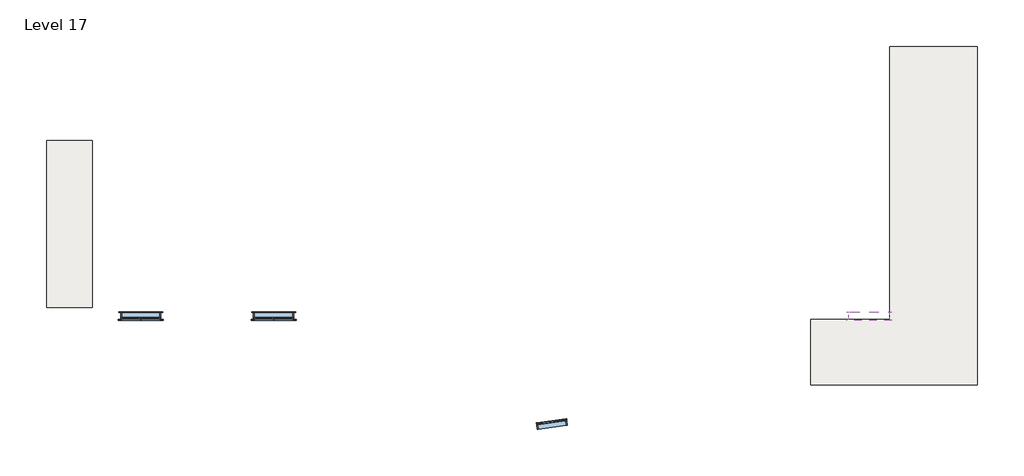
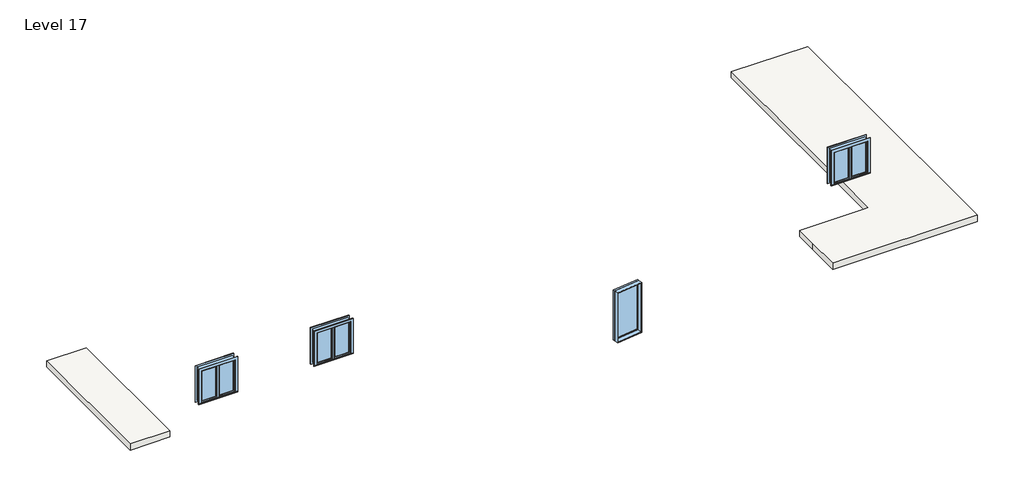
# One storey: 4 windows, 2 slabs.
"""IFC4 building model written with IfcOpenShell, lengths in millimetres."""

from ifc_helpers import new_model, si_unit, frame, origin, place, context, project, spatial, polyline, outline, extrude, transform, mapped, element, save
from components import window_0862ab64, window_9a779fa2

model = new_model("IFC4")

# Units and contexts
model_context = context("Model", 3, world=origin())
ifc_project = project(units=[si_unit("LENGTHUNIT", "METRE", prefix="MILLI")], contexts=[model_context])

# Site, building, storey
site = spatial("IfcSite", under=ifc_project)
building = spatial("IfcBuilding", under=site)
storey = spatial("IfcBuildingStorey", under=building, Name="Level 17", Elevation=26212.8)

# Slabs
placement = place(None, origin())
element("IfcSlab", 1, ObjectType="9\"", at=placement, inside=storey, context=model_context, shape_type="SweptSolid", body=[
    extrude(outline(polyline([(-17972.8272291, -8690.0239591), (-16601.2272291, -8690.0239591), (-16601.2272291, -13719.2239591), (-17972.8272291, -13719.2239591), (-17972.8272291, -8690.0239591)])), frame((0.0, 0.0, 25984.2), z_axis=(0.0, 0.0, 1.0), x_axis=(1.0, 0.0, 0.0)), (0.0, 0.0, 1.0), 228.6),
])
element("IfcSlab", 2, ObjectType="9\"", at=placement, inside=storey, context=model_context, shape_type="SweptSolid", body=[
    extrude(outline(polyline([(5046.5618272, -14840.0808221), (5046.5618272, -14078.0808221), (7230.9618272, -14078.0808221), (7434.1618272, -14078.0808221), (7434.1618272, -5848.4808221), (10075.7618272, -5848.4808221), (10075.7618272, -14840.0808221), (10075.7618272, -16059.2808221), (5046.5618272, -16059.2808221), (5046.5618272, -14840.0808221)])), frame((0.0, 0.0, 25984.2), z_axis=(0.0, 0.0, 1.0), x_axis=(1.0, 0.0, 0.0)), (0.0, 0.0, 1.0), 228.6),
])

# Windows
window_shape = window_0862ab64(model_context)
element("IfcWindow", 3, ObjectType="Casement Dbl with Trim : 48\" x 48\"", at=placement, inside=storey, context=model_context, shape_type="MappedRepresentation", body=[
    mapped(window_shape, transform((-15134.7505427, -13957.4308221, 26212.8), x_axis=(-1.0, 0.0, 0.0), y_axis=(0.0, -1.0, 0.0), z_axis=(0.0, 0.0, 1.0))),
])
element("IfcWindow", 4, ObjectType="Casement Dbl with Trim : 48\" x 48\"", at=placement, inside=storey, context=model_context, shape_type="MappedRepresentation", body=[
    mapped(window_shape, transform((-11129.6382271, -13957.4308221, 26212.8), x_axis=(-1.0, 0.0, 0.0), y_axis=(0.0, -1.0, 0.0), z_axis=(0.0, 0.0, 1.0))),
])
element("IfcWindow", 5, ObjectType="Casement Dbl with Trim : 48\" x 48\"", at=placement, inside=storey, context=model_context, shape_type="MappedRepresentation", body=[
    mapped(window_shape, transform((6810.8494573, -13957.4308221, 26558.0136494), x_axis=(-1.0, 0.0, 0.0), y_axis=(0.0, -1.0, 0.0), z_axis=(0.0, 0.0, 1.0))),
])
window_2_shape = window_9a779fa2(model_context)
element("IfcWindow", 6, ObjectType="Fixed : 36\" x 72\"", at=placement, inside=storey, context=model_context, shape_type="MappedRepresentation", body=[
    mapped(window_2_shape, transform((-2706.5288562, -17230.3159241, 26668.6120119), x_axis=(0.9910941253485877, 0.133163188229773, 0.0), y_axis=(-0.133163188229773, 0.9910941253485877, 0.0), z_axis=(0.0, 0.0, 1.0))),
])

save(model, "model.ifc")

# Revit data of these elements
# Type "9\""
#   Assembly Code = "B1010"
#   Function = 0
#   Layers, outside or top first: 0' - 9" no material (function 1)
# Type "Casement Dbl with Trim : 48\" x 48\""
#   Type Mark = "10"
#   Construction Type Id = "GSP4R"
#   Assembly Code = "B2020100"
#   Analytic Construction = "1/8 in Pilkington single glazing"
#   Visual Light Transmittance = 0.9
#   Solar Heat Gain Coefficient = 0.78
#   Heat Transfer Coefficient (U) = 0.6496 BTU/(h·ft²·°F)
#   Height = 4' - 0"
#   Default Sill Height = 3' - 0"
#   Trim Projection - Ext. = 0' - 0 1/2"
#   Trim Projection - Int. = 0' - 0 3/4"
#   Trim Width - Exterior = 0' - 3 1/2"
#   Trim Width - Interior = 0' - 3 1/2"
#   Width = 4' - 0"
#   Window Inset = 0' - 0 3/4"
#   Define Thermal Properties by = 1
#   Glass Pane Material = Glass
#   Sash Material = Sash
#   Trim Exterior Material = Trim
#   Trim Interior Material = Trim
#   Wall Closure = (empty or 0)
# Type "Fixed : 36\" x 72\""
#   Type Mark = "9"
#   Construction Type Id = "GSP4R"
#   Assembly Code = "B2020100"
#   Analytic Construction = "1/8 in Pilkington single glazing"
#   Visual Light Transmittance = 0.9
#   Solar Heat Gain Coefficient = 0.78
#   Heat Transfer Coefficient (U) = 0.6496 BTU/(h·ft²·°F)
#   Height = 6' - 0"
#   Default Sill Height = 1' - 0"
#   Width = 3' - 0"
#   Window Inset = 0' - 0 3/4"
#   Define Thermal Properties by = 1
#   Glass Pane Material = Glass
#   Sash Material = Sash
#   Wall Closure = (empty or 0)
# Element 1 (IfcSlab, "9\"")
#   built-in parameter 1001955 = 3.14159 (stored number, unit not read)
#   Height Offset From Level = 0' - 0"
#   Phase Created = New Construction
#   Materials on its faces: "Default Floor"
# Element 2 (IfcSlab, "9\"")
#   built-in parameter 1001955 = -1.5708 (stored number, unit not read)
#   Height Offset From Level = 0' - 0"
#   Phase Created = New Construction
#   Materials on its faces: "Default Floor"
# Element 3 (IfcWindow, "Casement Dbl with Trim : 48\" x 48\"")
#   Mark = "31"
#   Phase Created = New Construction
#   Materials on its faces: "Sash", "Trim", "Glass"
# Element 4 (IfcWindow, "Casement Dbl with Trim : 48\" x 48\"")
#   Mark = "32"
#   Phase Created = New Construction
#   Materials on its faces: "Sash", "Trim", "Glass"
# Element 5 (IfcWindow, "Casement Dbl with Trim : 48\" x 48\"")
#   Mark = "53"
#   Phase Created = New Construction
#   Materials on its faces: "Sash", "Trim", "Glass"
# Element 6 (IfcWindow, "Fixed : 36\" x 72\"")
#   Mark = "8"
#   Phase Created = New Construction
#   Materials on its faces: "Sash", "Glass"
# Materials
#   "Glass": class "Glass", colour RGB 0 128 192, transparency 0.75, Description = "Soda Lime Glass", Cost = 0
#   "Sash": class "Wood", colour RGB 224 178 126, transparency 0
#   "Trim": class "Wood", colour RGB 224 178 126, transparency 0
#   "Default Floor": colour RGB 128 128 128, transparency 0
